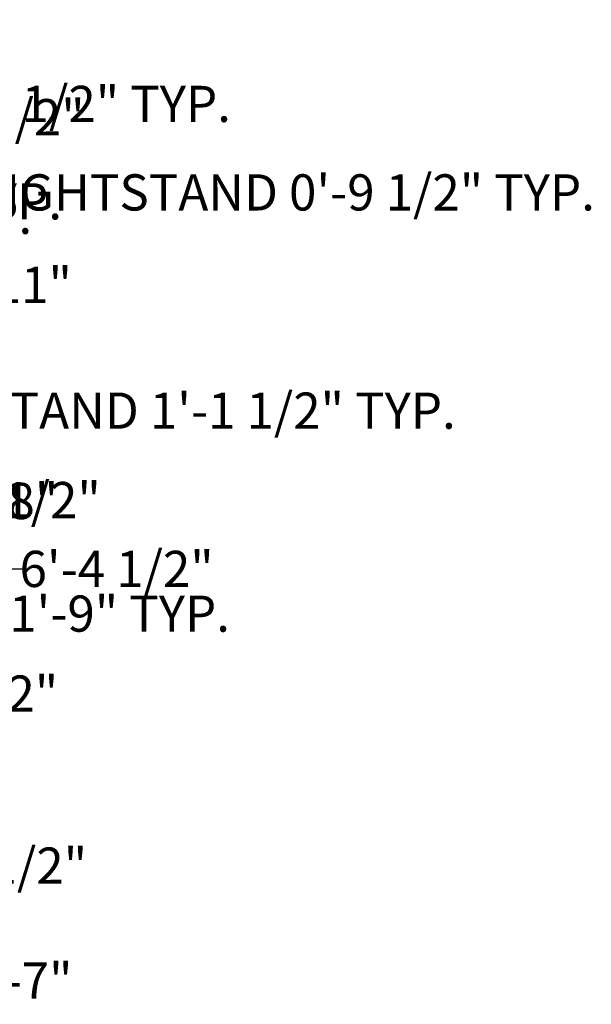
# Model space of a CAD drawing. Units: inches. Extents: x 29 to 6336, y 3 to 2592.
# Tile 8 of 8: x 5938 to 6336, y 1906 to 2590. Entities that reach past the tile are written whole.
import ezdxf

# ---------------------------------------------------------------- set-up
doc = ezdxf.new("R2010")
doc.units = ezdxf.units.IN
doc.header["$MEASUREMENT"] = 0
doc.layers.add('A-ANNO-DIMS', color=2, linetype='Continuous', lineweight=18)
doc.styles.get("Standard").update_dxf_attribs({"font": 'arial.ttf'})
doc.dimstyles.get("Standard").update_dxf_attribs({"dimtxt": 25.18, "dimasz": 25.18, "dimexe": 0.18, "dimexo": 0.0625, "dimgap": 0.09, "dimtad": 0, "dimtih": 1, "dimtoh": 1, "dimdec": 0, "dimzin": 0, "dimdsep": 46, "dimlunit": 3, "dimtxsty": 'Standard', "dimcen": 0.09, "dimadec": 0, "dimazin": 0, "dimtfac": 1, "dimtdec": 0, "dimtofl": 0, "dimtmove": 0, "dimatfit": 3, "dimfxl": 1, "dimtolj": 1, "dimtzin": 0, "dimarcsym": 0})

# ---------------------------------------------------------------- blocks, each defined once
blk = doc.blocks.new('*D30')
at = {"layer": 'A-ANNO-DIMS', "color": 0, "lineweight": -2, "transparency": 16777216}
for p, q in [((5810.39, 2470.26), (5785.21, 2470.26)), ((5835.57, 2471.66), (5835.57, 2470.08)), ((5845.31, 2471.66), (5845.31, 2470.08)), ((5870.49, 2470.26), (5895.67, 2470.26))]:
    blk.add_line(p, q, dxfattribs=at)
at = {"layer": 'A-ANNO-DIMS', "color": 0, "transparency": 16777216}
for points in [[(5810.39, 2474.46), (5810.39, 2466.06), (5835.57, 2470.26)], [(5870.49, 2474.46), (5870.49, 2466.06), (5845.31, 2470.26)]]:
    blk.add_solid(points, dxfattribs=at)
at = {"layer": 'Defpoints', "color": 0, "transparency": 16777216}
for p in [(5835.57, 2471.72), (5845.31, 2471.72), (5845.31, 2470.26)]:
    blk.add_point(p, dxfattribs=at)
at = {"layer": 'A-ANNO-DIMS', "color": 0, "transparency": 16777216, "insert": (6120.44, 2470.26), "char_height": 25.18, "attachment_point": 5}
blk.add_mtext('\\A1;NIGHTSTAND 0\'-9 1/2" TYP.', dxfattribs=at)
blk = doc.blocks.new('*D31')
at = {"layer": 'A-ANNO-DIMS', "color": 0, "lineweight": -2, "transparency": 16777216}
for p, q in [((5846.78, 2506.64), (5846.78, 2531.82)), ((5846.78, 2531.82), (5871.96, 2531.82)), ((5845.38, 2481.46), (5846.96, 2481.46)), ((5845.38, 2471.72), (5846.96, 2471.72)), ((5846.78, 2446.54), (5846.78, 2421.36))]:
    blk.add_line(p, q, dxfattribs=at)
at = {"layer": 'A-ANNO-DIMS', "color": 0, "transparency": 16777216}
for points in [[(5842.58, 2506.64), (5850.97, 2506.64), (5846.78, 2481.46)], [(5842.58, 2446.54), (5850.97, 2446.54), (5846.78, 2471.72)]]:
    blk.add_solid(points, dxfattribs=at)
at = {"layer": 'Defpoints', "color": 0, "transparency": 16777216}
for p in [(5845.31, 2481.46), (5846.78, 2481.46), (5845.31, 2471.72)]:
    blk.add_point(p, dxfattribs=at)
at = {"layer": 'A-ANNO-DIMS', "color": 0, "transparency": 16777216, "insert": (5978.13, 2531.82), "char_height": 25.18, "attachment_point": 5}
blk.add_mtext('\\A1;0\'-9 1/2" TYP.', dxfattribs=at)
blk = doc.blocks.new('*D32')
at = {"layer": 'A-ANNO-DIMS', "color": 0, "lineweight": -2, "transparency": 16777216}
for p, q in [((5709.84, 2318.47), (5684.66, 2318.47)), ((5735.02, 2316.52), (5735.02, 2318.65)), ((5748.43, 2316.52), (5748.43, 2318.65)), ((5773.61, 2318.47), (5798.79, 2318.47))]:
    blk.add_line(p, q, dxfattribs=at)
at = {"layer": 'A-ANNO-DIMS', "color": 0, "transparency": 16777216}
for points in [[(5709.84, 2322.67), (5709.84, 2314.27), (5735.02, 2318.47)], [(5773.61, 2322.67), (5773.61, 2314.27), (5748.43, 2318.47)]]:
    blk.add_solid(points, dxfattribs=at)
at = {"layer": 'Defpoints', "color": 0, "transparency": 16777216}
for p in [(5735.02, 2316.46), (5748.43, 2318.47), (5748.43, 2316.46)]:
    blk.add_point(p, dxfattribs=at)
at = {"layer": 'A-ANNO-DIMS', "color": 0, "transparency": 16777216, "insert": (6023.56, 2318.47), "char_height": 25.18, "attachment_point": 5}
blk.add_mtext('\\A1;NIGHTSTAND 1\'-1 1/2" TYP.', dxfattribs=at)
blk = doc.blocks.new('*D34')
at = {"layer": 'A-ANNO-DIMS', "color": 0, "lineweight": -2, "transparency": 16777216}
for p, q in [((5638.44, 2177.3), (5613.26, 2177.3)), ((5663.62, 2174.24), (5663.62, 2177.48)), ((5684.43, 2174.24), (5684.43, 2177.48)), ((5709.61, 2177.3), (5734.79, 2177.3))]:
    blk.add_line(p, q, dxfattribs=at)
at = {"layer": 'A-ANNO-DIMS', "color": 0, "transparency": 16777216}
for points in [[(5638.44, 2181.49), (5638.44, 2173.1), (5663.62, 2177.3)], [(5709.61, 2181.49), (5709.61, 2173.1), (5684.43, 2177.3)]]:
    blk.add_solid(points, dxfattribs=at)
at = {"layer": 'Defpoints', "color": 0, "transparency": 16777216}
for p in [(5663.62, 2174.18), (5684.43, 2177.3), (5684.43, 2174.18)]:
    blk.add_point(p, dxfattribs=at)
at = {"layer": 'A-ANNO-DIMS', "color": 0, "transparency": 16777216, "insert": (5913.59, 2177.3), "char_height": 25.18, "attachment_point": 5}
blk.add_mtext('\\A1;END TABLE 1\'-9" TYP.', dxfattribs=at)
blk = doc.blocks.new('*D36')
at = {"layer": 'A-ANNO-DIMS', "color": 0, "lineweight": -2, "transparency": 16777216}
for p, q in [((5520.77, 2458.79), (5520.77, 2453.82)), ((5553.13, 2458.79), (5553.13, 2453.82)), ((5495.59, 2454), (5470.41, 2454)), ((5578.31, 2454), (5603.49, 2454))]:
    blk.add_line(p, q, dxfattribs=at)
at = {"layer": 'A-ANNO-DIMS', "color": 0, "transparency": 16777216}
for points in [[(5495.59, 2458.2), (5495.59, 2449.81), (5520.77, 2454)], [(5578.31, 2458.2), (5578.31, 2449.81), (5553.13, 2454)]]:
    blk.add_solid(points, dxfattribs=at)
at = {"layer": 'Defpoints', "color": 0, "transparency": 16777216}
for p in [(5520.77, 2458.86), (5553.13, 2458.86), (5553.13, 2454)]:
    blk.add_point(p, dxfattribs=at)
at = {"layer": 'A-ANNO-DIMS', "color": 0, "transparency": 16777216, "insert": (5778.73, 2454), "char_height": 25.18, "attachment_point": 5}
blk.add_mtext('\\A1;VANITY 2\'-8 1/2" TYP.', dxfattribs=at)
blk = doc.blocks.new('*D40')
at = {"layer": 'A-ANNO-DIMS', "color": 0, "lineweight": -2, "transparency": 16777216}
for p, q in [((5460.58, 2466.07), (5460.58, 2463.89)), ((5474.29, 2466.07), (5474.29, 2463.89)), ((5435.4, 2464.07), (5410.22, 2464.07)), ((5499.47, 2464.07), (5524.65, 2464.07))]:
    blk.add_line(p, q, dxfattribs=at)
at = {"layer": 'A-ANNO-DIMS', "color": 0, "transparency": 16777216}
for points in [[(5435.4, 2468.27), (5435.4, 2459.88), (5460.58, 2464.07)], [(5499.47, 2468.27), (5499.47, 2459.88), (5474.29, 2464.07)]]:
    blk.add_solid(points, dxfattribs=at)
at = {"layer": 'Defpoints', "color": 0, "transparency": 16777216}
for p in [(5460.58, 2466.13), (5474.29, 2466.13), (5474.29, 2464.07)]:
    blk.add_point(p, dxfattribs=at)
at = {"layer": 'A-ANNO-DIMS', "color": 0, "transparency": 16777216, "insert": (5749.42, 2464.07), "char_height": 25.18, "attachment_point": 5}
blk.add_mtext('\\A1;NIGHTSTAND 1\'-1 1/2" TYP.', dxfattribs=at)
blk = doc.blocks.new('*D46')
at = {"layer": 'A-ANNO-DIMS', "color": 0, "lineweight": -2, "transparency": 16777216}
for p, q in [((5877.72, 2483.33), (5917.09, 2483.33)), ((5916.91, 2458.15), (5916.91, 2418.68)), ((5916.91, 2353.74), (5916.91, 2393.21)), ((5877.72, 2328.56), (5917.09, 2328.56))]:
    blk.add_line(p, q, dxfattribs=at)
at = {"layer": 'A-ANNO-DIMS', "color": 0, "transparency": 16777216}
for points in [[(5912.71, 2458.15), (5921.1, 2458.15), (5916.91, 2483.33)], [(5912.71, 2353.74), (5921.1, 2353.74), (5916.91, 2328.56)]]:
    blk.add_solid(points, dxfattribs=at)
at = {"layer": 'Defpoints', "color": 0, "transparency": 16777216}
for p in [(5877.66, 2483.33), (5916.91, 2483.33), (5877.66, 2328.56)]:
    blk.add_point(p, dxfattribs=at)
at = {"layer": 'A-ANNO-DIMS', "color": 0, "transparency": 16777216, "insert": (5916.91, 2405.95), "char_height": 25.18, "attachment_point": 5}
blk.add_mtext('\\A1;12\'-11"', dxfattribs=at)
blk = doc.blocks.new('*D50')
at = {"layer": 'A-ANNO-DIMS', "color": 0, "lineweight": -2, "transparency": 16777216}
for p, q in [((5510.17, 2319.56), (5917.09, 2319.56)), ((5916.91, 2294.38), (5916.91, 2268.55)), ((5916.91, 2216.83), (5916.91, 2242.66)), ((5510.17, 2191.65), (5917.09, 2191.65))]:
    blk.add_line(p, q, dxfattribs=at)
at = {"layer": 'A-ANNO-DIMS', "color": 0, "transparency": 16777216}
for points in [[(5912.71, 2294.38), (5921.1, 2294.38), (5916.91, 2319.56)], [(5912.71, 2216.83), (5921.1, 2216.83), (5916.91, 2191.65)]]:
    blk.add_solid(points, dxfattribs=at)
at = {"layer": 'Defpoints', "color": 0, "transparency": 16777216}
for p in [(5510.11, 2319.56), (5916.91, 2319.56), (5510.11, 2191.65)]:
    blk.add_point(p, dxfattribs=at)
at = {"layer": 'A-ANNO-DIMS', "color": 0, "transparency": 16777216, "insert": (5916.91, 2255.61), "char_height": 25.18, "attachment_point": 5}
blk.add_mtext('\\A1;10\'-8"', dxfattribs=at)
blk = doc.blocks.new('*D51')
at = {"layer": 'A-ANNO-DIMS', "color": 0, "lineweight": -2, "transparency": 16777216}
for p, q in [((5877.72, 2319.56), (5917.09, 2319.56)), ((5916.91, 2294.38), (5916.91, 2269.37)), ((5916.91, 2218.13), (5916.91, 2243.15)), ((5877.72, 2192.95), (5917.09, 2192.95))]:
    blk.add_line(p, q, dxfattribs=at)
at = {"layer": 'A-ANNO-DIMS', "color": 0, "transparency": 16777216}
for points in [[(5912.71, 2294.38), (5921.1, 2294.38), (5916.91, 2319.56)], [(5912.71, 2218.13), (5921.1, 2218.13), (5916.91, 2192.95)]]:
    blk.add_solid(points, dxfattribs=at)
at = {"layer": 'Defpoints', "color": 0, "transparency": 16777216}
for p in [(5877.66, 2319.56), (5916.91, 2319.56), (5877.66, 2192.95)]:
    blk.add_point(p, dxfattribs=at)
at = {"layer": 'A-ANNO-DIMS', "color": 0, "transparency": 16777216, "insert": (5916.91, 2256.26), "char_height": 25.18, "attachment_point": 5}
blk.add_mtext('\\A1;10\'-6 1/2"', dxfattribs=at)
blk = doc.blocks.new('*D53')
at = {"layer": 'A-ANNO-DIMS', "color": 0, "lineweight": -2, "transparency": 16777216}
for p, q in [((5801.82, 2182.65), (5917.09, 2182.65)), ((5916.91, 2157.47), (5916.91, 2134.63)), ((5916.91, 2085.9), (5916.91, 2108.74)), ((5801.82, 2060.72), (5917.09, 2060.72))]:
    blk.add_line(p, q, dxfattribs=at)
at = {"layer": 'A-ANNO-DIMS', "color": 0, "transparency": 16777216}
for points in [[(5912.71, 2157.47), (5921.1, 2157.47), (5916.91, 2182.65)], [(5912.71, 2085.9), (5921.1, 2085.9), (5916.91, 2060.72)]]:
    blk.add_solid(points, dxfattribs=at)
at = {"layer": 'Defpoints', "color": 0, "transparency": 16777216}
for p in [(5801.76, 2182.65), (5916.91, 2182.65), (5801.76, 2060.72)]:
    blk.add_point(p, dxfattribs=at)
at = {"layer": 'A-ANNO-DIMS', "color": 0, "transparency": 16777216, "insert": (5916.91, 2121.68), "char_height": 25.18, "attachment_point": 5}
blk.add_mtext('\\A1;10\'-2"', dxfattribs=at)
blk = doc.blocks.new('*D54')
at = {"layer": 'A-ANNO-DIMS', "color": 0, "lineweight": -2, "transparency": 16777216}
for p, q in [((5916.91, 2183.22), (5916.91, 2208.4)), ((5916.91, 2208.4), (5942.09, 2208.4)), ((5877.72, 2183.22), (5917.09, 2183.22)), ((5916.91, 2131.66), (5916.91, 2158.04)), ((5877.72, 2106.48), (5917.09, 2106.48))]:
    blk.add_line(p, q, dxfattribs=at)
at = {"layer": 'A-ANNO-DIMS', "color": 0, "transparency": 16777216}
for points in [[(5912.71, 2158.04), (5921.1, 2158.04), (5916.91, 2183.22)], [(5912.71, 2131.66), (5921.1, 2131.66), (5916.91, 2106.48)]]:
    blk.add_solid(points, dxfattribs=at)
at = {"layer": 'Defpoints', "color": 0, "transparency": 16777216}
for p in [(5877.66, 2183.22), (5916.91, 2183.22), (5877.66, 2106.48)]:
    blk.add_point(p, dxfattribs=at)
at = {"layer": 'A-ANNO-DIMS', "color": 0, "transparency": 16777216, "insert": (6005.05, 2208.4), "char_height": 25.18, "attachment_point": 5}
blk.add_mtext('\\A1;6\'-4 1/2"', dxfattribs=at)
blk = doc.blocks.new('*D55')
at = {"layer": 'A-ANNO-DIMS', "color": 0, "lineweight": -2, "transparency": 16777216}
for p, q in [((5810.76, 2106.42), (5810.76, 1921.9)), ((5877.66, 2106.42), (5877.66, 1921.9)), ((5835.94, 1922.08), (5852.48, 1922.08)), ((5877.66, 1922.08), (5902.84, 1922.08))]:
    blk.add_line(p, q, dxfattribs=at)
at = {"layer": 'A-ANNO-DIMS', "color": 0, "transparency": 16777216}
for points in [[(5835.94, 1926.28), (5835.94, 1917.88), (5810.76, 1922.08)], [(5852.48, 1926.28), (5852.48, 1917.88), (5877.66, 1922.08)]]:
    blk.add_solid(points, dxfattribs=at)
at = {"layer": 'Defpoints', "color": 0, "transparency": 16777216}
for p in [(5810.76, 2106.48), (5877.66, 2106.48), (5877.66, 1922.08)]:
    blk.add_point(p, dxfattribs=at)
at = {"layer": 'A-ANNO-DIMS', "color": 0, "transparency": 16777216, "insert": (5936.39, 1922.08), "char_height": 25.18, "attachment_point": 5}
blk.add_mtext('\\A1;5\'-7"', dxfattribs=at)
blk = doc.blocks.new('*D61')
at = {"layer": 'A-ANNO-DIMS', "color": 0, "lineweight": -2, "transparency": 16777216}
for p, q in [((5810.82, 2051.72), (5917.09, 2051.72)), ((5916.91, 2026.54), (5916.91, 2015.14)), ((5916.91, 1977.51), (5916.91, 1988.91)), ((5877.72, 1952.33), (5917.09, 1952.33))]:
    blk.add_line(p, q, dxfattribs=at)
at = {"layer": 'A-ANNO-DIMS', "color": 0, "transparency": 16777216}
for points in [[(5912.71, 2026.54), (5921.1, 2026.54), (5916.91, 2051.72)], [(5912.71, 1977.51), (5921.1, 1977.51), (5916.91, 1952.33)]]:
    blk.add_solid(points, dxfattribs=at)
at = {"layer": 'Defpoints', "color": 0, "transparency": 16777216}
for p in [(5810.76, 2051.72), (5877.66, 1952.33), (5916.91, 1952.33)]:
    blk.add_point(p, dxfattribs=at)
at = {"layer": 'A-ANNO-DIMS', "color": 0, "transparency": 16777216, "insert": (5916.91, 2002.02), "char_height": 25.18, "attachment_point": 5}
blk.add_mtext('\\A1;8\'-3 1/2"', dxfattribs=at)
blk = doc.blocks.new('*D67')
at = {"layer": 'A-ANNO-DIMS', "color": 0, "lineweight": -2, "transparency": 16777216}
for p, q in [((5743.99, 2522.58), (5718.81, 2522.58)), ((5769.17, 2150.03), (5769.17, 2522.76)), ((5801.76, 2182.71), (5801.76, 2522.76)), ((5826.94, 2522.58), (5852.12, 2522.58))]:
    blk.add_line(p, q, dxfattribs=at)
at = {"layer": 'A-ANNO-DIMS', "color": 0, "transparency": 16777216}
for points in [[(5743.99, 2526.78), (5743.99, 2518.38), (5769.17, 2522.58)], [(5826.94, 2526.78), (5826.94, 2518.38), (5801.76, 2522.58)]]:
    blk.add_solid(points, dxfattribs=at)
at = {"layer": 'Defpoints', "color": 0, "transparency": 16777216}
for p in [(5801.76, 2522.58), (5801.76, 2182.65), (5769.17, 2149.97)]:
    blk.add_point(p, dxfattribs=at)
at = {"layer": 'A-ANNO-DIMS', "color": 0, "transparency": 16777216, "insert": (5915.23, 2522.58), "char_height": 25.18, "attachment_point": 5}
blk.add_mtext('\\A1;2\'-8 1/2"', dxfattribs=at)

msp = doc.modelspace()

# ---------------------------------------------------------------- dimensions: what is measured, and where the dimension line sits
at = {"layer": 'A-ANNO-DIMS'}
dim = msp.add_linear_dim(base=(5846.78, 2481.46), p1=(5845.31, 2471.72), p2=(5845.31, 2481.46), angle=90, text='<> TYP.', dimstyle='Standard', override={"dimdec": 1, "dimlfac": 1, "dimrnd": 0, "dimzin": 1, "dimdsep": 46, "dimlunit": 4, "dimfrac": 2}, dxfattribs=at)
dim.commit()
dim.dimension.update_dxf_attribs({"geometry": '*D31', "text_midpoint": (5978.13, 2531.82)})
for base, p1, p2, picture, middle in [((5801.76, 2522.58), (5769.17, 2149.97), (5801.76, 2182.65), '*D67', (5915.23, 2522.58)), ((5877.66, 1922.08), (5810.76, 2106.48), (5877.66, 2106.48), '*D55', (5936.39, 1922.08))]:
    dim = msp.add_linear_dim(base=base, p1=p1, p2=p2, dimstyle='Standard', override={"dimdec": 1, "dimlfac": 1, "dimrnd": 0, "dimzin": 1, "dimdsep": 46, "dimlunit": 4, "dimfrac": 2}, dxfattribs=at)
    dim.commit()
    dim.dimension.update_dxf_attribs({"geometry": picture, "text_midpoint": middle})
for base, p1, p2, text, picture, middle in [((5845.31, 2470.26), (5835.57, 2471.72), (5845.31, 2471.72), 'NIGHTSTAND <> TYP.', '*D30', (6120.44, 2470.26)), ((5474.29, 2464.07), (5460.58, 2466.13), (5474.29, 2466.13), 'NIGHTSTAND <> TYP.', '*D40', (5749.42, 2464.07)), ((5553.13, 2454), (5520.77, 2458.86), (5553.13, 2458.86), 'VANITY <> TYP.', '*D36', (5778.73, 2454)), ((5748.43, 2318.47), (5735.02, 2316.46), (5748.43, 2316.46), 'NIGHTSTAND <> TYP.', '*D32', (6023.56, 2318.47)), ((5684.43, 2177.3), (5663.62, 2174.18), (5684.43, 2174.18), 'END TABLE <> TYP.', '*D34', (5913.59, 2177.3))]:
    dim = msp.add_linear_dim(base=base, p1=p1, p2=p2, text=text, dimstyle='Standard', override={"dimdec": 1, "dimlfac": 1, "dimrnd": 0, "dimzin": 1, "dimdsep": 46, "dimlunit": 4, "dimfrac": 2}, dxfattribs=at)
    dim.commit()
    dim.dimension.update_dxf_attribs({"geometry": picture, "text_midpoint": middle})
for base, p1, p2, picture, middle in [((5916.91, 2483.33), (5877.66, 2328.56), (5877.66, 2483.33), '*D46', (5916.91, 2405.95)), ((5916.91, 2319.56), (5510.11, 2191.65), (5510.11, 2319.56), '*D50', (5916.91, 2255.61)), ((5916.91, 2319.56), (5877.66, 2192.95), (5877.66, 2319.56), '*D51', (5916.91, 2256.26)), ((5916.91, 2183.22), (5877.66, 2106.48), (5877.66, 2183.22), '*D54', (6005.05, 2208.4)), ((5916.91, 2182.65), (5801.76, 2060.72), (5801.76, 2182.65), '*D53', (5916.91, 2121.68)), ((5916.91, 1952.33), (5810.76, 2051.72), (5877.66, 1952.33), '*D61', (5916.91, 2002.02))]:
    dim = msp.add_linear_dim(base=base, p1=p1, p2=p2, angle=90, dimstyle='Standard', override={"dimdec": 1, "dimlfac": 1, "dimrnd": 0, "dimzin": 1, "dimdsep": 46, "dimlunit": 4, "dimfrac": 2}, dxfattribs=at)
    dim.commit()
    dim.dimension.update_dxf_attribs({"geometry": picture, "text_midpoint": middle})

doc.saveas('drawing.dxf')
